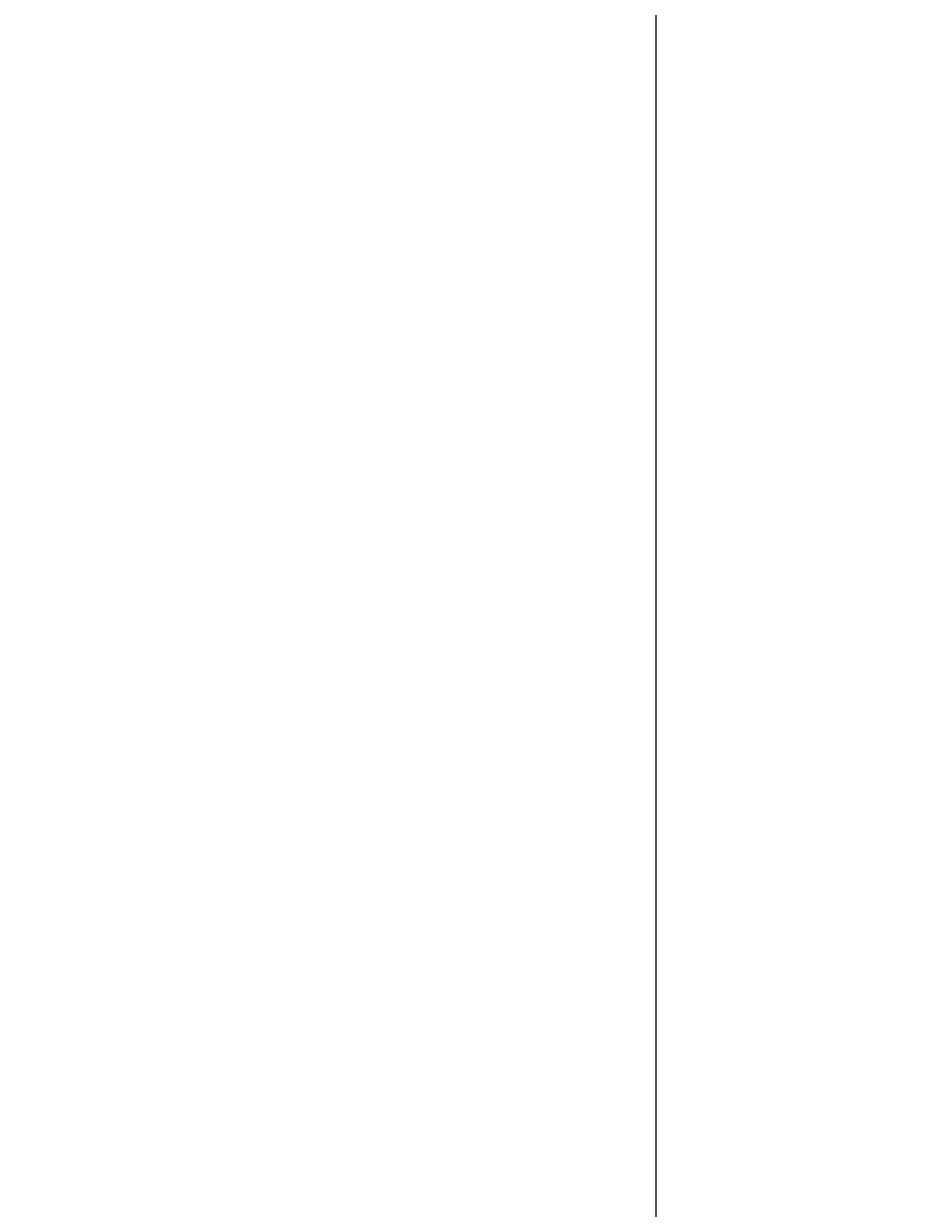
# Model space of a CAD drawing. Units: millimetres. Extents: x -11 to 280, y -4 to 208.
# Tile 39 of 55: x 244 to 266, y 55 to 85. Entities that reach past the tile are written whole.
import ezdxf

# ---------------------------------------------------------------- set-up
doc = ezdxf.new("R2010")
doc.units = ezdxf.units.MM
doc.layers.add('M-DIMS', color=2, linetype='Continuous', lineweight=18)
doc.styles.get("Standard").update_dxf_attribs({"font": 'arial.ttf'})
doc.dimstyles.get("Standard").update_dxf_attribs({"dimtxt": 0.18, "dimasz": 0.18, "dimexe": 0.18, "dimexo": 0.0625, "dimgap": 0.09, "dimtad": 0, "dimtih": 1, "dimtoh": 1, "dimdec": 4, "dimzin": 0, "dimdsep": 46, "dimtxsty": 'Standard', "dimcen": 0.09, "dimadec": 0, "dimazin": 0, "dimtfac": 1, "dimtdec": 4, "dimtofl": 0, "dimtmove": 0, "dimatfit": 3, "dimfxl": 1, "dimtolj": 1, "dimtzin": 0, "dimarcsym": 0})

# ---------------------------------------------------------------- blocks, each defined once
blk = doc.blocks.new('*D4')
at = {"layer": 'Defpoints', "color": 0, "transparency": 16777216}
for p in [(4.763, 84.426), (266.035, 51.733), (266.035, -3.415)]:
    blk.add_point(p, dxfattribs=at)
at = {"layer": 'M-DIMS', "color": 0, "lineweight": -2, "transparency": 16777216}
for p, q in [((4.763, 84.364), (4.763, -3.595)), ((266.035, 51.67), (266.035, -3.595)), ((4.943, -3.415), (134.934, -3.415)), ((265.855, -3.415), (135.864, -3.415))]:
    blk.add_line(p, q, dxfattribs=at)
at = {"layer": 'M-DIMS', "color": 0, "transparency": 16777216}
for points in [[(4.943, -3.385), (4.943, -3.445), (4.763, -3.415)], [(265.855, -3.385), (265.855, -3.445), (266.035, -3.415)]]:
    blk.add_solid(points, dxfattribs=at)
at = {"layer": 'M-DIMS', "color": 0, "transparency": 16777216, "insert": (135.399, -3.415), "char_height": 0.18, "attachment_point": 5}
blk.add_mtext('\\A1;261.27', dxfattribs=at)
blk = doc.blocks.new('*D5')
at = {"layer": 'Defpoints', "color": 0, "transparency": 16777216}
for p in [(24.759, 192.645), (-10.087, 11.435), (261.686, 11.435)]:
    blk.add_point(p, dxfattribs=at)
at = {"layer": 'M-DIMS', "color": 0, "lineweight": -2, "transparency": 16777216}
for p, q in [((24.696, 192.645), (-10.267, 192.645)), ((-10.087, 192.465), (-10.087, 102.222)), ((-10.087, 11.615), (-10.087, 101.858)), ((261.624, 11.435), (-10.267, 11.435))]:
    blk.add_line(p, q, dxfattribs=at)
at = {"layer": 'M-DIMS', "color": 0, "transparency": 16777216}
for points in [[(-10.117, 192.465), (-10.057, 192.465), (-10.087, 192.645)], [(-10.117, 11.615), (-10.057, 11.615), (-10.087, 11.435)]]:
    blk.add_solid(points, dxfattribs=at)
at = {"layer": 'M-DIMS', "color": 0, "transparency": 16777216, "insert": (-10.087, 102.04), "char_height": 0.18, "attachment_point": 5}
blk.add_mtext('\\A1;181.2', dxfattribs=at)
blk = doc.blocks.new('*D22')
at = {"layer": 'Defpoints', "color": 0, "transparency": 16777216}
for p in [(259.871, 207.495), (231.68, 34.723), (259.871, 34.723)]:
    blk.add_point(p, dxfattribs=at)
at = {"layer": 'M-DIMS', "color": 0, "lineweight": -2, "transparency": 16777216}
for p, q in [((231.68, 34.785), (231.68, 207.675)), ((259.871, 34.785), (259.871, 207.675)), ((231.86, 207.495), (245.38, 207.495)), ((259.691, 207.495), (246.171, 207.495))]:
    blk.add_line(p, q, dxfattribs=at)
at = {"layer": 'M-DIMS', "color": 0, "transparency": 16777216}
for points in [[(231.86, 207.525), (231.86, 207.465), (231.68, 207.495)], [(259.691, 207.525), (259.691, 207.465), (259.871, 207.495)]]:
    blk.add_solid(points, dxfattribs=at)
at = {"layer": 'M-DIMS', "color": 0, "transparency": 16777216, "insert": (245.776, 207.495), "char_height": 0.18, "attachment_point": 5}
blk.add_mtext('\\A1;28.19', dxfattribs=at)

msp = doc.modelspace()

# ---------------------------------------------------------------- dimensions: what is measured, and where the dimension line sits
at = {"layer": 'M-DIMS'}
for base, p1, p2, picture, middle in [((259.871, 207.495), (231.6803, 34.7226), (259.871, 34.7226), '*D22', (245.7757, 207.495)), ((266.0352, -3.4154), (4.7635, 84.4261), (266.0352, 51.7328), '*D4', (135.3993, -3.4154))]:
    dim = msp.add_linear_dim(base=base, p1=p1, p2=p2, dimstyle='Standard', override={"dimdec": 2, "dimlfac": 1, "dimrnd": 0, "dimzin": 0, "dimdsep": 46, "dimlunit": 2}, dxfattribs=at)
    dim.commit()
    dim.dimension.update_dxf_attribs({"geometry": picture, "text_midpoint": middle})
dim = msp.add_linear_dim(base=(-10.0865, 11.4346), p1=(24.7588, 192.645), p2=(261.6863, 11.4346), angle=90, dimstyle='Standard', override={"dimdec": 1, "dimlfac": 1, "dimrnd": 0, "dimzin": 0, "dimdsep": 46, "dimlunit": 2}, dxfattribs=at)
dim.commit()
dim.dimension.update_dxf_attribs({"geometry": '*D5', "text_midpoint": (-10.0865, 102.0398)})

doc.saveas('drawing.dxf')
